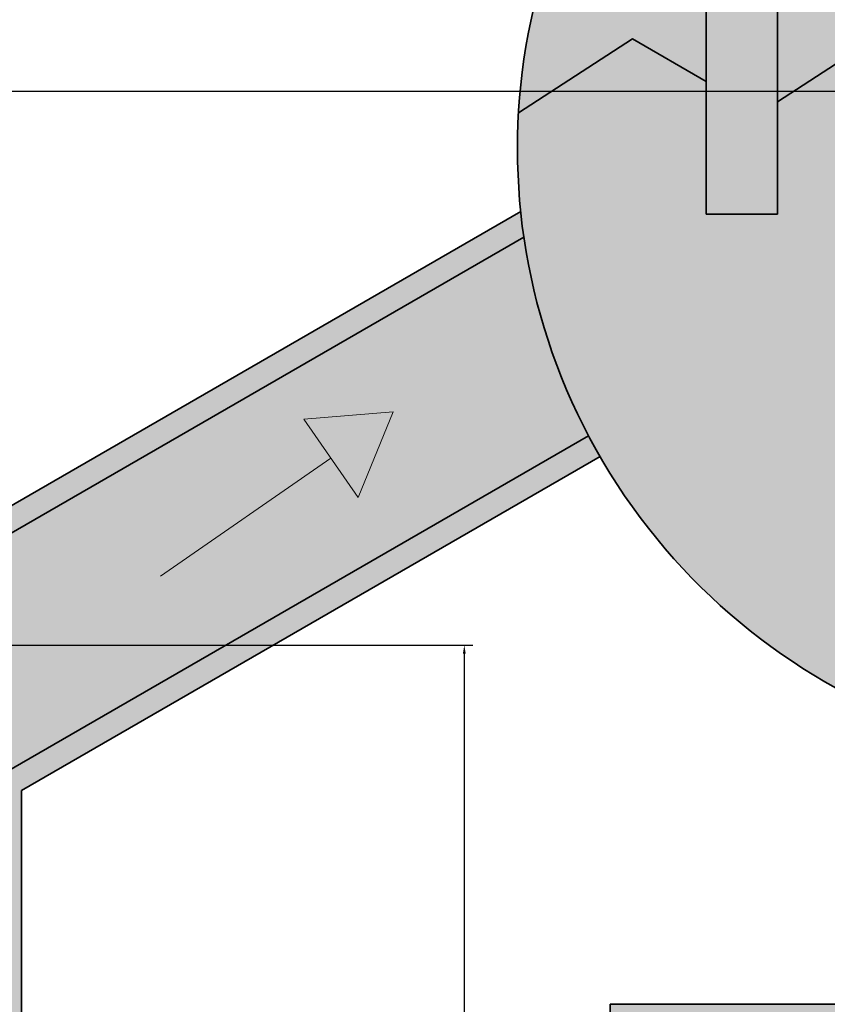
# Model space of a CAD drawing. Units: inches. Extents: x -1 to 292, y -3 to 199.
# Tile 46 of 52: x 220.5 to 237.47, y 80.58 to 101.27. Entities that reach past the tile are written whole.
import ezdxf

# ---------------------------------------------------------------- set-up
doc = ezdxf.new("R2010")
doc.units = ezdxf.units.IN
doc.header["$MEASUREMENT"] = 0
for name, color, linetype, lineweight in [('M-ANNO-SYMB', 1, 'Continuous', 18), ('M-DIMS', 2, 'Continuous', 18), ('M-EQPM', 7, 'Continuous', 35), ('M-PATT', 8, 'Continuous', 13)]:
    doc.layers.add(name, color=color, linetype=linetype, lineweight=lineweight)
doc.styles.get("Standard").update_dxf_attribs({"font": 'arial.ttf'})
doc.dimstyles.get("Standard").update_dxf_attribs({"dimtxt": 0.18, "dimasz": 0.18, "dimexe": 0.18, "dimexo": 0.0625, "dimgap": 0.09, "dimtad": 0, "dimtih": 1, "dimtoh": 1, "dimdec": 4, "dimzin": 0, "dimdsep": 46, "dimtxsty": 'Standard', "dimcen": 0.09, "dimadec": 0, "dimazin": 0, "dimtfac": 1, "dimtdec": 4, "dimtofl": 0, "dimtmove": 0, "dimatfit": 3, "dimfxl": 1, "dimtolj": 1, "dimtzin": 0, "dimarcsym": 0})

# ---------------------------------------------------------------- blocks, each defined once
blk = doc.blocks.new('FLOW-ARROW-WATER')
blk.add_line((223.29, 53.741), (227.063, 51.564))
blk.add_lwpolyline([(222.79, 52.875), (221.849, 54.506), (223.79, 54.608)], close=True)
blk = doc.blocks.new('*D10')
at = {"layer": 'Defpoints', "color": 0, "transparency": 16777216}
for p in [(169.176, 99.774), (169.176, 43.391), (292.04, 43.391)]:
    blk.add_point(p, dxfattribs=at)
at = {"layer": 'M-DIMS', "color": 0, "lineweight": -2, "transparency": 16777216}
for p, q in [((169.239, 99.774), (292.22, 99.774)), ((292.04, 99.594), (292.04, 71.764)), ((292.04, 43.571), (292.04, 71.4)), ((169.239, 43.391), (292.22, 43.391))]:
    blk.add_line(p, q, dxfattribs=at)
at = {"layer": 'M-DIMS', "color": 0, "transparency": 16777216}
for points in [[(292.01, 99.594), (292.07, 99.594), (292.04, 99.774)], [(292.01, 43.571), (292.07, 43.571), (292.04, 43.391)]]:
    blk.add_solid(points, dxfattribs=at)
at = {"layer": 'M-DIMS', "color": 0, "transparency": 16777216, "insert": (292.04, 71.582), "char_height": 0.18, "attachment_point": 5}
blk.add_mtext('\\A1;56.38', dxfattribs=at)
blk = doc.blocks.new('*D25')
at = {"layer": 'Defpoints', "color": 0, "transparency": 16777216}
for p in [(273.066, 88.419), (215.241, 88.13), (273.066, -2.71)]:
    blk.add_point(p, dxfattribs=at)
at = {"layer": 'M-DIMS', "color": 0, "lineweight": -2, "transparency": 16777216}
for p, q in [((273.066, 88.357), (273.066, -2.89)), ((215.241, 88.068), (215.241, -2.89)), ((215.421, -2.71), (243.76, -2.71)), ((272.886, -2.71), (244.547, -2.71))]:
    blk.add_line(p, q, dxfattribs=at)
at = {"layer": 'M-DIMS', "color": 0, "transparency": 16777216}
for points in [[(215.421, -2.68), (215.421, -2.74), (215.241, -2.71)], [(272.886, -2.68), (272.886, -2.74), (273.066, -2.71)]]:
    blk.add_solid(points, dxfattribs=at)
at = {"layer": 'M-DIMS', "color": 0, "transparency": 16777216, "insert": (244.153, -2.71), "char_height": 0.18, "attachment_point": 5}
blk.add_mtext('\\A1;57.83', dxfattribs=at)
blk = doc.blocks.new('*D26')
at = {"layer": 'Defpoints', "color": 0, "transparency": 16777216}
for p in [(215.241, 88.13), (215.241, 55.034), (229.841, 55.034)]:
    blk.add_point(p, dxfattribs=at)
at = {"layer": 'M-DIMS', "color": 0, "lineweight": -2, "transparency": 16777216}
for p, q in [((215.303, 88.13), (230.021, 88.13)), ((229.841, 87.95), (229.841, 71.764)), ((229.841, 55.214), (229.841, 71.4)), ((215.303, 55.034), (230.021, 55.034))]:
    blk.add_line(p, q, dxfattribs=at)
at = {"layer": 'M-DIMS', "color": 0, "transparency": 16777216}
for points in [[(229.811, 87.95), (229.871, 87.95), (229.841, 88.13)], [(229.811, 55.214), (229.871, 55.214), (229.841, 55.034)]]:
    blk.add_solid(points, dxfattribs=at)
at = {"layer": 'M-DIMS', "color": 0, "transparency": 16777216, "insert": (229.841, 71.582), "char_height": 0.18, "attachment_point": 5}
blk.add_mtext('\\A1;33.1', dxfattribs=at)

msp = doc.modelspace()

# ---------------------------------------------------------------- hatches: boundary and pattern name
at = {"layer": 'M-PATT'}
h = msp.add_hatch(color=256, dxfattribs=at)
h.set_gradient(color1=(0, 127, 0), color2=(0, 127, 0), tint=1, name='CYLINDER')
h.paths.add_polyline_path([(164.5186, 119.2985), (129.9293, 119.2985), (129.9293, 117.2985), (164.1897, 117.2985)])
h.paths.add_polyline_path([(181.5897, 119.2985), (164.5186, 119.2985), (164.1897, 117.2985), (179.5897, 117.2985), (179.5897, 107.8518), (181.5897, 109.1506)])
h.paths.add_polyline_path([(181.5897, 109.1506), (179.5897, 107.8518), (179.5897, 36.2698), (198.4159, 36.2698), (198.4159, 38.2698), (181.5897, 38.2698)])
h.paths.add_polyline_path([(115.4883, 126.765), (111.4883, 126.765), (111.4883, 114.6589), (115.4883, 114.6589)])
h.paths.add_polyline_path([(123.408, 119.2985), (115.4883, 119.2985), (115.4883, 117.2985), (123.408, 117.2985)])
h.paths.add_polyline_path([(115.4883, 112.6589), (111.4883, 112.6589), (111.4883, 106.9941), (115.4883, 106.9941)])
h.paths.add_polyline_path([(120.9032, 106.9941), (106.0735, 106.9941), (106.0735, 105.9941), (120.9032, 105.9941)])
h.paths.add_polyline_path([(236.4209, 117.5104), (234.9209, 117.5104), (234.9209, 97.1861), (236.4209, 97.1861)])
h.paths.add_polyline_path([(236.4209, 126.4904), (234.9209, 126.4904), (234.9209, 118.9331), (236.4209, 118.9331)])
h.paths.add_polyline_path([(244.9552, 125.7269), (242.9552, 125.7269), (242.9552, 116.8562), (244.9552, 116.8562)])
h.paths.add_polyline_path([(244.9552, 115.1721), (242.9552, 115.1721), (242.9552, 109.7385), (244.9552, 109.7385)])
h.paths.add_polyline_path([(248.4468, 109.7385), (239.4637, 109.7385), (239.4637, 109.4289), (248.4468, 109.4289)])
h = msp.add_hatch(color=256, dxfattribs=at)
h.set_gradient(color1=(205, 32, 39), color2=(242, 113, 114), tint=1, name='CYLINDER')
h.paths.add_polyline_path([(243.5443, 100.87), (246.2365, 99.3157), (248.6299, 100.87), (251.3221, 99.3157), (253.7155, 100.87), (256.4077, 99.3157), (256.8092, 99.5764, 0.3682504), (244.9552, 111.4691), (244.9552, 109.7385), (248.4468, 109.7385), (248.4468, 107.2081), (239.4637, 107.2081), (239.4637, 109.7385), (242.9552, 109.7385), (242.9552, 111.4772, 0.1365835), (236.4209, 109.1305), (236.4209, 99.5466), (238.4587, 100.87), (241.1509, 99.3157)])
h.paths.add_polyline_path([(230.9797, 99.3157), (233.3731, 100.87), (234.9209, 99.9764), (234.9209, 107.8885, 0.1887049)])
h = msp.add_hatch(color=256, dxfattribs=at)
h.set_gradient(color1=(0, 255, 255), color2=(0, 255, 255), tint=1, name='CYLINDER')
h.paths.add_polyline_path([(256.8092, 99.5764), (256.4077, 99.3157), (253.7155, 100.87), (251.3221, 99.3157), (248.6299, 100.87), (246.2365, 99.3157), (243.5443, 100.87), (241.1509, 99.3157), (238.4587, 100.87), (236.4209, 99.5466), (236.4209, 97.1861), (234.9209, 97.1861), (234.9209, 99.9764), (233.3731, 100.87), (230.9797, 99.3157, 1.0704128)])
h.paths.add_polyline_path([(234.4549, 44.5975, 1), (253.3518, 44.5975, 1)])
h.paths.add_polyline_path([(235.4822, 48.8821), (220.034, 57.8011), (220.034, 85.363), (232.4507, 92.5318, -0.0853739), (231.0925, 96.7051), (215.7407, 87.8418), (215.7407, 55.3224), (234.4552, 44.5176, -0.0021162), (234.4549, 44.5975, -0.1182098)])
h.paths.add_polyline_path([(222.7904, 52.8755), (221.8492, 54.5058), (223.7904, 54.6075)], flags=16)
h.paths.add_polyline_path([(216.828, 66.8912), (217.7692, 68.5216), (218.828, 66.8912)], flags=16)
h.paths.add_polyline_path([(216.8084, 83.826), (217.7497, 85.4564), (218.8084, 83.826)], flags=16)
h.paths.add_polyline_path([(226.468, 92.8803), (228.3442, 93.0348), (227.6068, 91.2362)], flags=16)
h.paths.add_polyline_path([(272.5659, 88.1304), (260.2765, 95.2257), (259.0113, 93.0196), (263.0639, 91.1046), (263.4912, 92.0087), (264.5631, 90.4612), (262.6367, 90.2004), (263.0639, 91.1046), (259.0113, 93.0196), (257.8918, 91.0677), (267.7726, 85.363), (267.7726, 57.8011), (255.5043, 50.718), (257.0663, 46.085), (272.5659, 55.0337)])
h.paths.add_polyline_path([(263.6286, 51.5636), (261.7461, 51.5636), (262.6286, 53.2956)], flags=16)
h.paths.add_polyline_path([(269.8773, 65.3608), (268.8186, 66.9911), (270.8186, 66.9911)], flags=16)
h.paths.add_polyline_path([(269.8773, 80.8843), (268.8186, 82.5146), (270.8186, 82.5146)], flags=16)
h.paths.add_polyline_path([(255.5043, 50.718), (252.3244, 48.8821, -0.1182098), (253.3518, 44.5975, -0.0177685), (253.3279, 43.9266), (257.0663, 46.085)])
h.paths.add_polyline_path([(260.2765, 95.2257), (256.7809, 97.2439, -0.0959457), (255.356, 92.5318), (257.8918, 91.0677)])
h = msp.add_hatch(color=256, dxfattribs=at)
h.set_gradient(color1=(76, 38, 47), color2=(76, 38, 47), tint=1, name='CYLINDER')
h.paths.add_polyline_path([(267.2726, 58.0898), (255.3414, 51.2013), (255.5043, 50.718), (267.7726, 57.8011), (267.7726, 85.363), (257.8918, 91.0677), (257.643, 90.634), (267.2726, 85.0743)])
h.paths.add_polyline_path([(272.5659, 55.0337), (257.0663, 46.085), (257.2293, 45.6017), (273.0659, 54.745), (273.0659, 88.4191), (260.5253, 95.6595), (260.2765, 95.2257), (272.5659, 88.1304)])
h.paths.add_polyline_path([(215.2407, 55.0337), (234.4787, 43.9266, -0.0156517), (234.4552, 44.5176), (215.7407, 55.3224), (215.7407, 87.8418), (231.0925, 96.7051, -0.0104859), (231.0257, 97.2439), (215.2407, 88.1304)])
h.paths.add_polyline_path([(220.034, 57.8011), (235.4822, 48.8821, -0.0132367), (235.7207, 49.3218), (220.534, 58.0898), (220.534, 85.0743), (232.6923, 92.0939, -0.0096587), (232.4507, 92.5318), (220.034, 85.363)])
h = msp.add_hatch(color=256, dxfattribs=at)
h.set_gradient(color1=(0, 0, 255), color2=(0, 0, 255), tint=1, name='CYLINDER')
h.paths.add_polyline_path([(227.6068, 91.2362), (228.3442, 93.0348), (226.468, 92.8803)])
h.paths.add_polyline_path([(218.8084, 83.826), (217.7497, 85.4564), (216.8084, 83.826)])
h.paths.add_polyline_path([(262.6367, 90.2004), (264.5631, 90.4612), (263.4912, 92.0087)])
h.paths.add_polyline_path([(217.7692, 68.5216), (216.828, 66.8912), (218.828, 66.8912)])
h.paths.add_polyline_path([(223.7904, 54.6075), (221.8492, 54.5058), (222.7904, 52.8755)])
h.paths.add_polyline_path([(262.6286, 53.2956), (261.7461, 51.5636), (263.6286, 51.5636)])
h.paths.add_polyline_path([(268.8186, 82.5146), (269.8773, 80.8843), (270.8186, 82.5146)])
h.paths.add_polyline_path([(268.8186, 66.9911), (269.8773, 65.3608), (270.8186, 66.9911)])
h = msp.add_hatch(color=256, dxfattribs=at)
h.set_gradient(color1=(242, 103, 34), color2=(242, 103, 34), tint=1, name='CYLINDER')
h.paths.add_polyline_path([(232.9033, 62.5821), (254.9033, 62.5821), (254.9033, 80.5821), (251.8779, 80.5821), (250.2521, 77.7473), (252.0686, 77.7473), (252.0686, 65.4168), (235.7381, 65.4168), (235.7381, 77.7473), (250.2521, 77.7473), (251.8779, 80.5821), (232.9033, 80.5821)])

# ---------------------------------------------------------------- linework, layer by layer
at = {"layer": 'M-EQPM'}
for p, q in [((234.9209, 97.1861), (234.9209, 117.5104)), ((236.4209, 97.1861), (236.4209, 117.5104)), ((236.4209, 97.1861), (234.9209, 97.1861))]:
    msp.add_line(p, q, dxfattribs=at)
for points in [[(230.9797, 99.3157), (233.3731, 100.87), (234.9209, 99.9764)], [(236.4209, 99.5466), (238.4587, 100.87), (241.1509, 99.3157)], [(231.0257, 97.2439), (215.2407, 88.1304), (215.2407, 55.0337), (234.4787, 43.9266)], [(231.0925, 96.7051), (215.7407, 87.8418), (215.7407, 55.3224), (234.4552, 44.5176)], [(232.4507, 92.5318), (220.034, 85.363), (220.034, 57.8011), (235.4822, 48.8821)], [(232.6923, 92.0939), (220.534, 85.0743), (220.534, 58.0898), (235.7207, 49.3218)]]:
    msp.add_lwpolyline(points, dxfattribs=at)
msp.add_lwpolyline([(232.9033, 80.5821), (254.9033, 80.5821), (254.9033, 62.5821), (232.9033, 62.5821)], close=True, dxfattribs=at)
msp.add_arc((243.9033, 98.5666), 12.9453, 133.93743, 85.33905, dxfattribs=at)

# ---------------------------------------------------------------- block references
at = {"layer": 'M-ANNO-SYMB', "rotation": 244.7076562269448}
msp.add_blockref('FLOW-ARROW-WATER', (273.8455, 316.9044), dxfattribs=at)

# ---------------------------------------------------------------- dimensions: what is measured, and where the dimension line sits
at = {"layer": 'M-DIMS'}
for base, p1, p2, angle, override, picture, middle in [((292.0399, 43.3906), (169.176, 99.7735), (169.176, 43.3906), 90, {"dimdec": 2, "dimlfac": 1, "dimrnd": 0, "dimzin": 0, "dimdsep": 46, "dimlunit": 2}, '*D10', (292.0399, 71.5821)), ((229.8407, 55.0337), (215.2407, 88.1304), (215.2407, 55.0337), 270, {"dimdec": 1, "dimlfac": 1, "dimrnd": 0, "dimzin": 0, "dimdsep": 46, "dimlunit": 2}, '*D26', (229.8407, 71.5821))]:
    dim = msp.add_linear_dim(base=base, p1=p1, p2=p2, angle=angle, dimstyle='Standard', override=override, dxfattribs=at)
    dim.commit()
    dim.dimension.update_dxf_attribs({"geometry": picture, "text_midpoint": middle})
dim = msp.add_linear_dim(base=(273.0659, -2.7104), p1=(215.2407, 88.1304), p2=(273.0659, 88.4191), dimstyle='Standard', override={"dimdec": 2, "dimlfac": 1, "dimrnd": 0, "dimzin": 0, "dimdsep": 46, "dimlunit": 2}, dxfattribs=at)
dim.commit()
dim.dimension.update_dxf_attribs({"geometry": '*D25', "text_midpoint": (244.1533, -2.7104)})

doc.saveas('drawing.dxf')
